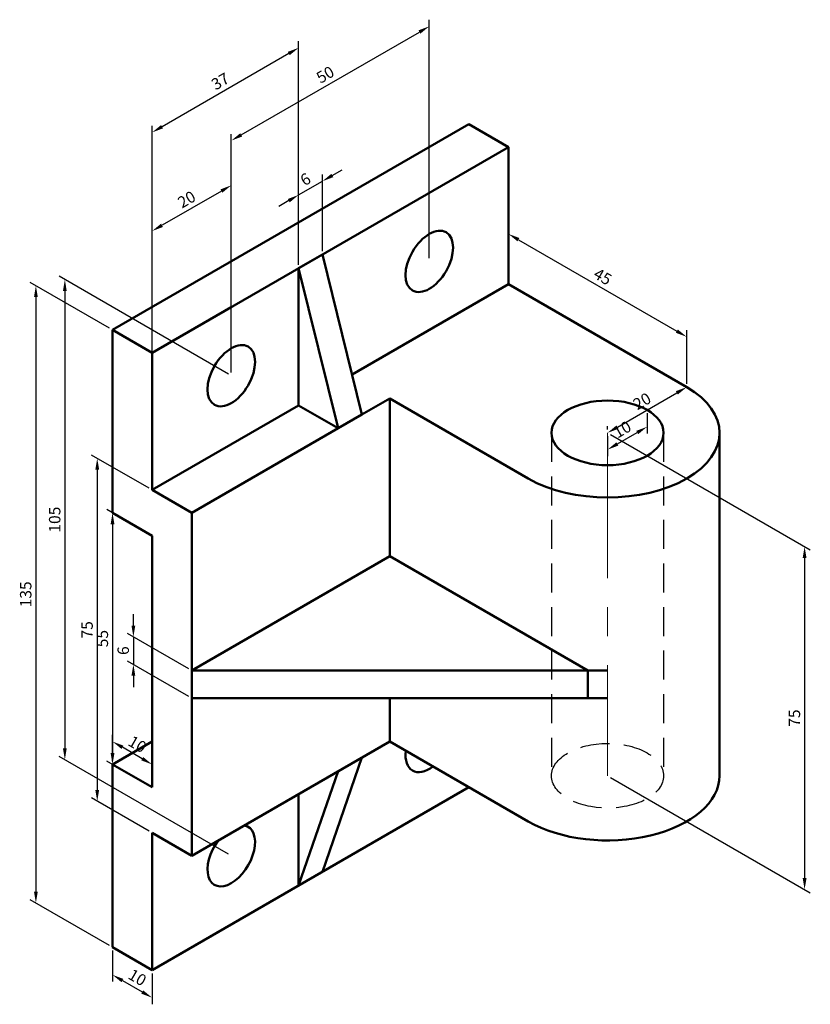
# Model space of a CAD drawing. Units: millimetres. Extents: x 83 to 256, y 32 to 247.
import ezdxf

# ---------------------------------------------------------------- set-up
doc = ezdxf.new("R2010")
doc.units = ezdxf.units.MM
doc.linetypes.add('CENTER', pattern=[50.8, 31.75, -6.35, 6.35, -6.35])
doc.linetypes.add('HIDDEN', pattern=[9.525, 6.35, -3.175])
for name, color, linetype, lineweight in [('M-CNTR', 1, 'CENTER', 18), ('M-DIMS', 2, 'Continuous', 25), ('M-HIDN', 4, 'HIDDEN', 25), ('M-OUTL', 7, 'Continuous', 50)]:
    doc.layers.add(name, color=color, linetype=linetype, lineweight=lineweight)
doc.styles.get("Standard").update_dxf_attribs({"font": 'arial.ttf'})
doc.dimstyles.new('ISO-25', dxfattribs={"dimtxt": 2.5, "dimasz": 2.5, "dimexe": 1.25, "dimexo": 0.625, "dimtad": 1, "dimtxsty": 'Standard', "dimcen": 2.5, "dimadec": 0, "dimazin": 0, "dimtfac": 1, "dimtmove": 0, "dimatfit": 3, "dimfxl": 1, "dimarcsym": 0})

# ---------------------------------------------------------------- blocks, each defined once
blk = doc.blocks.new('*D1')
at = {"layer": 'Defpoints', "color": 0, "transparency": 16777216}
for p in [(172.62, 245.56), (172.62, 194.14), (129.32, 169.14)]:
    blk.add_point(p, dxfattribs=at)
at = {"layer": 'M-DIMS', "color": 0, "lineweight": -2, "transparency": 16777216}
for p, q in [((172.62, 194.87), (172.62, 247)), ((131.49, 221.81), (170.46, 244.31)), ((129.32, 169.87), (129.32, 222))]:
    blk.add_line(p, q, dxfattribs=at)
at = {"layer": 'M-DIMS', "color": 0, "transparency": 16777216}
for points in [[(170.25, 244.67), (170.67, 243.95), (172.62, 245.56)], [(131.28, 222.17), (131.69, 221.45), (129.32, 220.56)]]:
    blk.add_solid(points, dxfattribs=at)
at = {"layer": 'M-DIMS', "color": 0, "transparency": 16777216, "insert": (150.02, 234.71), "char_height": 2.5, "attachment_point": 5, "rotation": 30}
blk.add_mtext('50', dxfattribs=at)
blk = doc.blocks.new('*D2')
at = {"layer": 'Defpoints', "color": 0, "transparency": 16777216}
for p in [(149.24, 211.68), (149.24, 195.64), (144.04, 192.64)]:
    blk.add_point(p, dxfattribs=at)
at = {"layer": 'M-DIMS', "color": 0, "lineweight": -2, "transparency": 16777216}
for p, q in [((151.4, 212.93), (153.57, 214.18)), ((144.04, 208.68), (149.24, 211.68)), ((149.24, 196.37), (149.24, 213.12)), ((144.04, 193.37), (144.04, 210.12)), ((141.88, 207.43), (139.71, 206.18))]:
    blk.add_line(p, q, dxfattribs=at)
at = {"layer": 'M-DIMS', "color": 0, "transparency": 16777216}
for points in [[(151.2, 213.29), (151.61, 212.56), (149.24, 211.68)], [(141.67, 207.79), (142.09, 207.06), (144.04, 208.68)]]:
    blk.add_solid(points, dxfattribs=at)
at = {"layer": 'M-DIMS', "color": 0, "transparency": 16777216, "insert": (145.69, 211.82), "char_height": 2.5, "attachment_point": 5, "rotation": 30}
blk.add_mtext('6', dxfattribs=at)
blk = doc.blocks.new('*D3')
at = {"layer": 'Defpoints', "color": 0, "transparency": 16777216}
for p in [(112, 200.78), (129.32, 169.14), (112, 159.14)]:
    blk.add_point(p, dxfattribs=at)
at = {"layer": 'M-DIMS', "color": 0, "lineweight": -2, "transparency": 16777216}
for p, q in [((129.32, 169.87), (129.32, 212.22)), ((127.16, 209.53), (114.17, 202.03)), ((112, 159.87), (112, 202.22))]:
    blk.add_line(p, q, dxfattribs=at)
at = {"layer": 'M-DIMS', "color": 0, "transparency": 16777216}
for points in [[(126.95, 209.89), (127.36, 209.17), (129.32, 210.78)], [(113.96, 202.39), (114.37, 201.67), (112, 200.78)]]:
    blk.add_solid(points, dxfattribs=at)
at = {"layer": 'M-DIMS', "color": 0, "transparency": 16777216, "insert": (119.71, 207.42), "char_height": 2.5, "attachment_point": 5, "rotation": 30}
blk.add_mtext('20', dxfattribs=at)
blk = doc.blocks.new('*D4')
at = {"layer": 'Defpoints', "color": 0, "transparency": 16777216}
for p in [(112, 222.35), (144.04, 192.64), (112, 174.14)]:
    blk.add_point(p, dxfattribs=at)
at = {"layer": 'M-DIMS', "color": 0, "lineweight": -2, "transparency": 16777216}
for p, q in [((144.04, 193.37), (144.04, 242.29)), ((141.88, 239.6), (114.17, 223.6)), ((112, 174.87), (112, 223.79))]:
    blk.add_line(p, q, dxfattribs=at)
at = {"layer": 'M-DIMS', "color": 0, "transparency": 16777216}
for points in [[(141.67, 239.96), (142.09, 239.24), (144.04, 240.85)], [(113.96, 223.96), (114.37, 223.24), (112, 222.35)]]:
    blk.add_solid(points, dxfattribs=at)
at = {"layer": 'M-DIMS', "color": 0, "transparency": 16777216, "insert": (127.07, 233.25), "char_height": 2.5, "attachment_point": 5, "rotation": 30}
blk.add_mtext('37', dxfattribs=at)
blk = doc.blocks.new('*D5')
at = {"layer": 'Defpoints', "color": 0, "transparency": 16777216}
for p in [(103.34, 179.14), (86.58, 53.82), (103.34, 44.14)]:
    blk.add_point(p, dxfattribs=at)
at = {"layer": 'M-DIMS', "color": 0, "lineweight": -2, "transparency": 16777216}
for p, q in [((102.71, 179.51), (85.33, 189.54)), ((86.58, 186.32), (86.58, 56.32)), ((102.71, 44.51), (85.33, 54.54))]:
    blk.add_line(p, q, dxfattribs=at)
at = {"layer": 'M-DIMS', "color": 0, "transparency": 16777216}
for points in [[(86.17, 186.32), (87, 186.32), (86.58, 188.82)], [(86.17, 56.32), (87, 56.32), (86.58, 53.82)]]:
    blk.add_solid(points, dxfattribs=at)
at = {"layer": 'M-DIMS', "color": 0, "transparency": 16777216, "insert": (84.68, 121.32), "char_height": 2.5, "attachment_point": 5, "rotation": 90}
blk.add_mtext('135', dxfattribs=at)
blk = doc.blocks.new('*D6')
at = {"layer": 'Defpoints', "color": 0, "transparency": 16777216}
for p in [(129.32, 169.14), (92.92, 85.16), (129.32, 64.14)]:
    blk.add_point(p, dxfattribs=at)
at = {"layer": 'M-DIMS', "color": 0, "lineweight": -2, "transparency": 16777216}
for p, q in [((128.7, 169.51), (91.67, 190.88)), ((92.92, 187.66), (92.92, 87.66)), ((128.7, 64.51), (91.67, 85.88))]:
    blk.add_line(p, q, dxfattribs=at)
at = {"layer": 'M-DIMS', "color": 0, "transparency": 16777216}
for points in [[(92.5, 187.66), (93.33, 187.66), (92.92, 190.16)], [(92.5, 87.66), (93.33, 87.66), (92.92, 85.16)]]:
    blk.add_solid(points, dxfattribs=at)
at = {"layer": 'M-DIMS', "color": 0, "transparency": 16777216, "insert": (91.02, 137.66), "char_height": 2.5, "attachment_point": 5, "rotation": 90}
blk.add_mtext('105', dxfattribs=at)
blk = doc.blocks.new('*D7')
at = {"layer": 'Defpoints', "color": 0, "transparency": 16777216}
for p in [(112, 144.14), (100, 76.07), (112, 69.14)]:
    blk.add_point(p, dxfattribs=at)
at = {"layer": 'M-DIMS', "color": 0, "lineweight": -2, "transparency": 16777216}
for p, q in [((111.37, 144.51), (98.75, 151.79)), ((100, 148.57), (100, 78.57)), ((111.37, 69.51), (98.75, 76.79))]:
    blk.add_line(p, q, dxfattribs=at)
at = {"layer": 'M-DIMS', "color": 0, "transparency": 16777216}
for points in [[(99.58, 148.57), (100.42, 148.57), (100, 151.07)], [(99.58, 78.57), (100.42, 78.57), (100, 76.07)]]:
    blk.add_solid(points, dxfattribs=at)
at = {"layer": 'M-DIMS', "color": 0, "transparency": 16777216, "insert": (98.1, 113.57), "char_height": 2.5, "attachment_point": 5, "rotation": 90}
blk.add_mtext('75', dxfattribs=at)
blk = doc.blocks.new('*D8')
at = {"layer": 'Defpoints', "color": 0, "transparency": 16777216}
for p in [(112, 134.14), (103.34, 84.14), (112, 79.14)]:
    blk.add_point(p, dxfattribs=at)
at = {"layer": 'M-DIMS', "color": 0, "lineweight": -2, "transparency": 16777216}
for p, q in [((111.37, 134.51), (102.09, 139.87)), ((103.34, 136.64), (103.34, 86.64)), ((111.37, 79.51), (102.09, 84.87))]:
    blk.add_line(p, q, dxfattribs=at)
at = {"layer": 'M-DIMS', "color": 0, "transparency": 16777216}
for points in [[(102.92, 136.64), (103.76, 136.64), (103.34, 139.14)], [(102.92, 86.64), (103.76, 86.64), (103.34, 84.14)]]:
    blk.add_solid(points, dxfattribs=at)
at = {"layer": 'M-DIMS', "color": 0, "transparency": 16777216, "insert": (101.44, 111.64), "char_height": 2.5, "attachment_point": 5, "rotation": 90}
blk.add_mtext('55', dxfattribs=at)
blk = doc.blocks.new('*D9')
at = {"layer": 'Defpoints', "color": 0, "transparency": 16777216}
for p in [(107.9, 106.01), (120.66, 104.64), (120.66, 98.64)]:
    blk.add_point(p, dxfattribs=at)
at = {"layer": 'M-DIMS', "color": 0, "lineweight": -2, "transparency": 16777216}
for p, q in [((107.9, 114.51), (107.9, 117.01)), ((120.04, 105.01), (106.65, 112.73)), ((107.9, 112.01), (107.9, 106.01)), ((120.04, 99.01), (106.65, 106.73)), ((107.9, 103.51), (107.9, 101.01))]:
    blk.add_line(p, q, dxfattribs=at)
at = {"layer": 'M-DIMS', "color": 0, "transparency": 16777216}
for points in [[(107.48, 114.51), (108.32, 114.51), (107.9, 112.01)], [(107.48, 103.51), (108.32, 103.51), (107.9, 106.01)]]:
    blk.add_solid(points, dxfattribs=at)
at = {"layer": 'M-DIMS', "color": 0, "transparency": 16777216, "insert": (106, 109.01), "char_height": 2.5, "attachment_point": 5, "rotation": 90}
blk.add_mtext('6', dxfattribs=at)
blk = doc.blocks.new('*D10')
at = {"layer": 'Defpoints', "color": 0, "transparency": 16777216}
for p in [(103.34, 44.14), (112, 39.14), (112, 33.11)]:
    blk.add_point(p, dxfattribs=at)
at = {"layer": 'M-DIMS', "color": 0, "lineweight": -2, "transparency": 16777216}
for p, q in [((103.34, 43.42), (103.34, 36.67)), ((105.5, 36.86), (109.83, 34.36)), ((112, 38.42), (112, 31.67))]:
    blk.add_line(p, q, dxfattribs=at)
at = {"layer": 'M-DIMS', "color": 0, "transparency": 16777216}
for points in [[(105.71, 37.22), (105.3, 36.5), (103.34, 38.11)], [(110.04, 34.72), (109.63, 34), (112, 33.11)]]:
    blk.add_solid(points, dxfattribs=at)
at = {"layer": 'M-DIMS', "color": 0, "transparency": 16777216, "insert": (108.62, 37.26), "char_height": 2.5, "attachment_point": 5, "rotation": 330}
blk.add_mtext('10', dxfattribs=at)
blk = doc.blocks.new('*D11')
at = {"layer": 'Defpoints', "color": 0, "transparency": 16777216}
for p in [(103.34, 89.13), (103.34, 84.14), (112, 79.14)]:
    blk.add_point(p, dxfattribs=at)
at = {"layer": 'M-DIMS', "color": 0, "lineweight": -2, "transparency": 16777216}
for p, q in [((103.34, 84.87), (103.34, 90.57)), ((109.83, 85.38), (105.5, 87.88)), ((112, 79.87), (112, 85.57))]:
    blk.add_line(p, q, dxfattribs=at)
at = {"layer": 'M-DIMS', "color": 0, "transparency": 16777216}
for points in [[(105.71, 88.24), (105.3, 87.52), (103.34, 89.13)], [(110.04, 85.74), (109.63, 85.02), (112, 84.13)]]:
    blk.add_solid(points, dxfattribs=at)
at = {"layer": 'M-DIMS', "color": 0, "transparency": 16777216, "insert": (108.62, 88.27), "char_height": 2.5, "attachment_point": 5, "rotation": 330}
blk.add_mtext('10', dxfattribs=at)
blk = doc.blocks.new('*D12')
at = {"layer": 'Defpoints', "color": 0, "transparency": 16777216}
for p in [(228.91, 166.64), (228.91, 166.64), (211.59, 156.64)]:
    blk.add_point(p, dxfattribs=at)
at = {"layer": 'M-DIMS', "color": 0, "lineweight": -2, "transparency": 16777216}
for p, q in [((228.91, 167.37), (228.91, 168.09)), ((213.76, 157.89), (226.75, 165.39)), ((211.59, 157.37), (211.59, 158.09))]:
    blk.add_line(p, q, dxfattribs=at)
at = {"layer": 'M-DIMS', "color": 0, "transparency": 16777216}
for points in [[(226.54, 165.76), (226.96, 165.03), (228.91, 166.64)], [(213.55, 158.26), (213.97, 157.53), (211.59, 156.64)]]:
    blk.add_solid(points, dxfattribs=at)
at = {"layer": 'M-DIMS', "color": 0, "transparency": 16777216, "insert": (219.3, 163.29), "char_height": 2.5, "attachment_point": 5, "rotation": 30}
blk.add_mtext('20', dxfattribs=at)
blk = doc.blocks.new('*D13')
at = {"layer": 'Defpoints', "color": 0, "transparency": 16777216}
for p in [(220.25, 161.64), (220.25, 157.97), (211.59, 156.64)]:
    blk.add_point(p, dxfattribs=at)
at = {"layer": 'M-DIMS', "color": 0, "lineweight": -2, "transparency": 16777216}
for p, q in [((220.25, 160.92), (220.25, 156.53)), ((211.59, 155.92), (211.59, 151.53)), ((213.76, 154.22), (218.09, 156.72))]:
    blk.add_line(p, q, dxfattribs=at)
at = {"layer": 'M-DIMS', "color": 0, "transparency": 16777216}
for points in [[(217.88, 157.08), (218.3, 156.36), (220.25, 157.97)], [(213.55, 154.58), (213.97, 153.86), (211.59, 152.97)]]:
    blk.add_solid(points, dxfattribs=at)
at = {"layer": 'M-DIMS', "color": 0, "transparency": 16777216, "insert": (214.97, 157.12), "char_height": 2.5, "attachment_point": 5, "rotation": 30}
blk.add_mtext('10', dxfattribs=at)
blk = doc.blocks.new('*D14')
at = {"layer": 'Defpoints', "color": 0, "transparency": 16777216}
for p in [(189.94, 189.14), (228.91, 177.64), (228.91, 166.64)]:
    blk.add_point(p, dxfattribs=at)
at = {"layer": 'M-DIMS', "color": 0, "lineweight": -2, "transparency": 16777216}
for p, q in [((189.94, 189.87), (189.94, 201.59)), ((192.11, 198.89), (226.75, 178.89)), ((228.91, 167.37), (228.91, 179.09))]:
    blk.add_line(p, q, dxfattribs=at)
at = {"layer": 'M-DIMS', "color": 0, "transparency": 16777216}
for points in [[(192.32, 199.25), (191.9, 198.53), (189.94, 200.14)], [(226.96, 179.25), (226.54, 178.53), (228.91, 177.64)]]:
    blk.add_solid(points, dxfattribs=at)
at = {"layer": 'M-DIMS', "color": 0, "transparency": 16777216, "insert": (210.38, 190.54), "char_height": 2.5, "attachment_point": 5, "rotation": 330}
blk.add_mtext('45', dxfattribs=at)
blk = doc.blocks.new('*D15')
at = {"layer": 'Defpoints', "color": 0, "transparency": 16777216}
for p in [(211.59, 156.64), (211.59, 81.64), (254.69, 56.76)]:
    blk.add_point(p, dxfattribs=at)
at = {"layer": 'M-DIMS', "color": 0, "lineweight": -2, "transparency": 16777216}
for p, q in [((212.22, 156.28), (255.94, 131.04)), ((254.69, 129.26), (254.69, 59.26)), ((212.22, 81.28), (255.94, 56.04))]:
    blk.add_line(p, q, dxfattribs=at)
at = {"layer": 'M-DIMS', "color": 0, "transparency": 16777216}
for points in [[(254.27, 129.26), (255.11, 129.26), (254.69, 131.76)], [(254.27, 59.26), (255.11, 59.26), (254.69, 56.76)]]:
    blk.add_solid(points, dxfattribs=at)
at = {"layer": 'M-DIMS', "color": 0, "transparency": 16777216, "insert": (252.79, 94.26), "char_height": 2.5, "attachment_point": 5, "rotation": 90}
blk.add_mtext('75', dxfattribs=at)

msp = doc.modelspace()

# ---------------------------------------------------------------- linework, layer by layer
at = {"layer": 'M-CNTR'}
msp.add_line((211.593, 156.645), (211.593, 81.645), dxfattribs=at)
at = {"layer": 'M-HIDN'}
for p, q in [((199.345, 156.645), (199.345, 81.645)), ((223.84, 156.645), (223.84, 81.645))]:
    msp.add_line(p, q, dxfattribs=at)
msp.add_ellipse((211.593, 81.645), major_axis=(-12.247, 0), ratio=0.5773503, dxfattribs=at)
at = {"layer": 'M-OUTL'}
for p, q in [((103.34, 179.145), (181.282, 224.145)), ((181.282, 224.145), (189.942, 219.145)), ((189.942, 219.145), (112, 174.145)), ((189.942, 219.145), (189.942, 189.145)), ((144.043, 192.645), (149.239, 195.645)), ((149.239, 195.645), (157.899, 160.645)), ((144.043, 162.645), (144.043, 192.645)), ((144.043, 192.645), (152.703, 157.645)), ((155.734, 169.395), (189.942, 189.145)), ((189.942, 189.145), (228.913, 166.645)), ((112, 174.145), (129.32, 184.145)), ((103.34, 179.145), (112, 174.145)), ((103.34, 179.145), (103.34, 139.145)), ((103.34, 139.145), (103.34, 179.145)), ((112, 174.145), (112, 144.145)), ((157.899, 160.645), (163.961, 164.145)), ((194.272, 146.645), (163.961, 164.145)), ((163.961, 164.145), (163.961, 129.645)), ((112, 144.145), (144.043, 162.645)), ((144.043, 162.645), (152.703, 157.645)), ((152.703, 157.645), (157.899, 160.645)), ((120.66, 139.145), (152.703, 157.645)), ((236.088, 156.645), (236.088, 81.645)), ((120.66, 139.145), (112, 144.145)), ((112, 134.145), (103.34, 139.145)), ((120.66, 101.645), (120.66, 139.145)), ((112, 106.645), (112, 134.145)), ((112, 134.145), (112, 79.145)), ((120.66, 104.645), (163.961, 129.645)), ((163.961, 129.645), (207.263, 104.645)), ((112, 106.645), (112, 79.145)), ((120.66, 104.645), (211.593, 104.645)), ((207.262, 98.645), (207.262, 104.645)), ((120.66, 101.645), (120.66, 64.145)), ((120.66, 98.645), (211.593, 98.645)), ((163.961, 89.145), (163.961, 98.645)), ((103.339, 84.145), (112, 89.145)), ((120.66, 64.145), (163.961, 89.145)), ((163.961, 89.145), (194.272, 71.645)), ((103.34, 44.145), (103.34, 84.145)), ((112, 79.145), (103.34, 84.145)), ((149.239, 60.645), (157.899, 85.645)), ((152.703, 82.645), (144.043, 57.645)), ((112, 39.145), (181.282, 79.145)), ((144.043, 77.645), (144.043, 57.645)), ((120.66, 64.145), (112, 69.145)), ((112, 69.145), (112, 39.145)), ((144.043, 57.645), (149.239, 60.645)), ((112, 39.145), (129.32, 49.145)), ((112, 39.145), (103.34, 44.145))]:
    msp.add_line(p, q, dxfattribs=at)
for centre, major_axis in [((172.622, 194.145), (-3.674, -6.364)), ((129.32, 169.145), (-3.674, -6.364)), ((211.593, 156.645), (-12.247, 0))]:
    msp.add_ellipse(centre, major_axis=major_axis, ratio=0.5773503, dxfattribs=at)
for centre, major_axis, start_param, end_param in [((211.593, 156.645), (-24.495, 0), 0.7853982, 3.9269908), ((172.621, 89.145), (3.674, 6.364), 2.2009336, 3.1415927), ((172.621, 89.145), (3.674, 6.364), 3.1415927, 4.0822517), ((211.593, 81.645), (-24.495, 0), 0.7853982, 3.1415927), ((129.32, 64.145), (-3.674, -6.364), 4.5126764, 9.6244906)]:
    msp.add_ellipse(centre, major_axis=major_axis, ratio=0.5773503, start_param=start_param, end_param=end_param, dxfattribs=at)

# ---------------------------------------------------------------- dimensions: what is measured, and where the dimension line sits
at = {"layer": 'M-DIMS'}
for p1, p2, distance, picture, middle in [((129.32, 169.145), (172.622, 194.145), 44.526, '*D1', (150.02, 234.705)), ((144.043, 192.645), (112, 174.145), -41.746, '*D4', (127.07, 233.246)), ((144.043, 192.645), (149.239, 195.645), 13.883, '*D2', (145.69, 211.822)), ((129.32, 169.145), (112, 159.145), -36.055, '*D3', (119.709, 207.424)), ((189.942, 189.145), (228.913, 166.645), 9.525, '*D14', (210.376, 190.535)), ((211.593, 156.645), (228.913, 166.645), 0, '*D12', (219.302, 163.292)), ((211.593, 156.645), (220.253, 161.645), -3.18, '*D13', (214.972, 157.119)), ((112, 79.145), (103.34, 84.145), -4.314, '*D11', (108.621, 88.273)), ((103.34, 44.145), (112, 39.145), -5.228, '*D10', (108.621, 37.255))]:
    dim = msp.add_aligned_dim(p1=p1, p2=p2, distance=distance, dimstyle='ISO-25', override={"dimclrd": 0, "dimclre": 0, "dimclrt": 0}, dxfattribs=at)
    dim.commit()
    dim.dimension.update_dxf_attribs({"geometry": picture, "text_midpoint": middle})
for base, p1, p2, picture, middle in [((86.583, 53.819), (103.34, 179.145), (103.34, 44.145), '*D5', (84.681, 121.319)), ((92.917, 85.163), (129.32, 169.145), (129.32, 64.145), '*D6', (91.015, 137.663)), ((254.689, 56.763), (211.593, 156.645), (211.593, 81.645), '*D15', (252.793, 94.263)), ((100.001, 76.072), (112, 144.145), (112, 69.145), '*D7', (98.105, 113.572)), ((103.34, 84.145), (112, 134.145), (112, 79.145), '*D8', (101.443, 111.645)), ((107.901, 106.011), (120.66, 104.645), (120.66, 98.645), '*D9', (106, 109.011))]:
    dim = msp.add_linear_dim(base=base, p1=p1, p2=p2, angle=90, dimstyle='ISO-25', override={"dimclrd": 0, "dimclre": 0, "dimclrt": 0}, dxfattribs=at)
    dim.commit()
    dim.dimension.update_dxf_attribs({"geometry": picture, "text_midpoint": middle})

doc.saveas('drawing.dxf')
